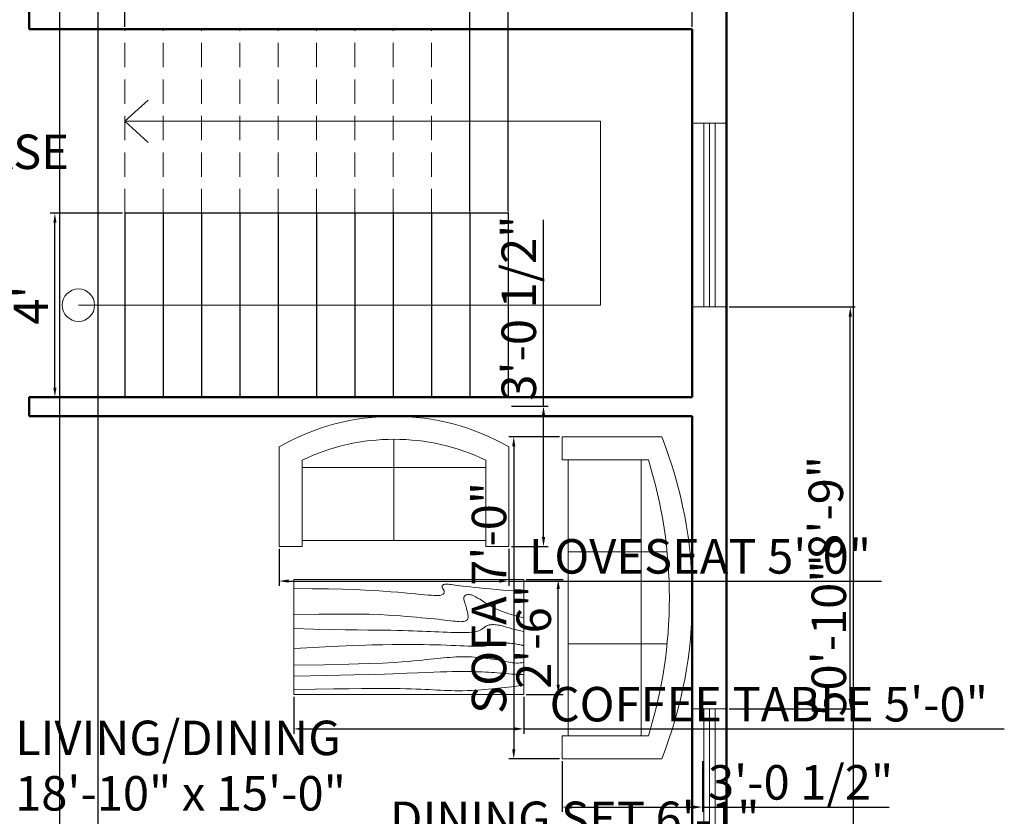
# Model space of a CAD drawing. Units: inches. Extents: x 2866 to 3545, y 873 to 1597.
# Tile 4 of 5: x 3239 to 3495, y 1172 to 1380. Entities that reach past the tile are written whole.
import ezdxf

# ---------------------------------------------------------------- set-up
doc = ezdxf.new("R2010")
doc.units = ezdxf.units.IN
doc.linetypes.add('HIDDEN', pattern=[9.525, 6.35, -3.175])
doc.layers.add('A-ANNO-DIMS', color=152, linetype='Continuous', lineweight=18, true_color=0x2776bb)
for name, color, linetype, lineweight in [('A-ANNO-SYMB', 7, 'Continuous', 18), ('A-AREA-IDEN', 7, 'Continuous', 25), ('A-FLOR-STRS', 7, 'Continuous', 25), ('A-FLOR-STRS-OVHD', 7, 'HIDDEN', 18), ('A-FURN', 8, 'Continuous', 18), ('A-GLAZ', 4, 'Continuous', 18), ('A-WALL', 7, 'Continuous', 50)]:
    doc.layers.add(name, color=color, linetype=linetype, lineweight=lineweight)
doc.styles.get("Standard").update_dxf_attribs({"font": 'arial.ttf'})
doc.dimstyles.new('ISO-25', dxfattribs={"dimtxt": 9, "dimasz": 2.5, "dimexe": 1.25, "dimexo": 0.625, "dimtad": 1, "dimdec": 0, "dimlunit": 3, "dimtxsty": 'Standard', "dimcen": 4.5, "dimadec": 0, "dimazin": 0, "dimtfac": 1, "dimtdec": 0, "dimtmove": 0, "dimatfit": 3, "dimfxl": 1, "dimarcsym": 0})

# ---------------------------------------------------------------- blocks, each defined once
blk = doc.blocks.new('Table - Rectangular Woodgrain 60 x 30 in.')
for p, q in [((0, 0), (0, -30)), ((60, 0), (0, 0)), ((60, -30), (60, 0)), ((0, -30), (60, -30))]:
    blk.add_line(p, q)
for points in [[(0, -2.4), (4.8155, -2.418), (9.0302, -2.4688), (12.709, -2.5477), (15.9167, -2.65), (18.7181, -2.7711), (21.1781, -2.9063), (23.3616, -3.0508), (25.3333, -3.2), (27.1477, -3.3495), (28.8172, -3.4958), (30.3437, -3.636), (31.7291, -3.7667), (32.9756, -3.8849), (34.0849, -3.9875), (35.059, -4.0714), (35.9, -4.1334), (36.6114, -4.1711), (37.2041, -4.1854), (37.6906, -4.1779), (38.0833, -4.15), (38.3948, -4.1034), (38.6375, -4.0396), (38.8239, -3.9602), (38.9666, -3.8667), (39.0764, -3.7608), (39.1573, -3.6448), (39.2116, -3.521), (39.2416, -3.3917), (39.2498, -3.2593), (39.2385, -3.1261), (39.21, -2.9944), (39.1666, -2.8667), (39.111, -2.7447), (39.0468, -2.6281), (38.978, -2.5163), (38.9083, -2.4083), (38.8418, -2.3035), (38.7823, -2.201), (38.7337, -2.1001), (38.7, -2), (38.6844, -1.9003), (38.6875, -1.8021), (38.7094, -1.707), (38.75, -1.6167), (38.8094, -1.5326), (38.8875, -1.4563), (38.9844, -1.3893), (39.1, -1.3333), (39.2351, -1.2896), (39.3937, -1.2583), (39.5804, -1.2396), (39.8, -1.2333), (40.057, -1.2396), (40.3562, -1.2583), (40.7023, -1.2896), (41.1, -1.3333), (41.5547, -1.3895), (42.0755, -1.4573), (42.6721, -1.5361), (43.3542, -1.625), (44.1316, -1.7233), (45.014, -1.8302), (46.0114, -1.9449), (47.1333, -2.0667), (48.3862, -2.1947), (49.7625, -2.3281), (51.2513, -2.4663), (52.8416, -2.6083), (54.5226, -2.7535), (56.2833, -2.9011), (58.1127, -3.0501), (60, -3.2)], [(0, -9.2), (6.5759, -9.0858), (11.9385, -9.0365), (16.2527, -9.0418), (19.6833, -9.0917), (22.3952, -9.1759), (24.5531, -9.2844), (26.322, -9.4069), (27.8666, -9.5333), (29.3241, -9.6553), (30.7203, -9.7719), (32.0532, -9.8837), (33.3208, -9.9917), (34.5213, -10.0965), (35.6526, -10.199), (36.7128, -10.2999), (37.7, -10.4), (38.6129, -10.4996), (39.4531, -10.5969), (40.223, -10.6895), (40.925, -10.775), (41.5613, -10.8512), (42.1344, -10.9156), (42.6465, -10.966), (43.1, -11), (43.4976, -11.0158), (43.8437, -11.0136), (44.143, -10.9942), (44.4, -10.9583), (44.6195, -10.9069), (44.8062, -10.8406), (44.9648, -10.7603), (45.1, -10.6667), (45.2155, -10.5598), (45.3114, -10.4365), (45.3871, -10.2929), (45.4416, -10.125), (45.4743, -9.929), (45.4844, -9.7011), (45.4709, -9.4371), (45.4333, -9.1333), (45.3716, -8.7883), (45.2896, -8.4104), (45.1919, -8.0107), (45.0833, -7.6), (44.9685, -7.1893), (44.8521, -6.7896), (44.7388, -6.4117), (44.6333, -6.0667), (44.54, -5.7628), (44.4614, -5.4979), (44.4001, -5.2675), (44.3583, -5.0667), (44.3384, -4.8909), (44.3427, -4.7354), (44.3736, -4.5956), (44.4333, -4.4667), (44.5236, -4.3453), (44.6427, -4.2333), (44.7884, -4.1339), (44.9583, -4.05), (45.1501, -3.9849), (45.3614, -3.9417), (45.59, -3.9234), (45.8333, -3.9333), (46.0915, -3.9749), (46.3734, -4.0531), (46.6906, -4.1736), (47.0542, -4.3417), (47.4756, -4.5629), (47.9661, -4.8427), (48.5372, -5.1866), (49.2, -5.6), (49.9676, -6.0844), (50.8594, -6.625), (51.8965, -7.2031), (53.1, -7.8), (54.491, -8.3969), (56.0906, -8.975), (57.9199, -9.5156), (60, -10)], [(0, -12.8), (5.1847, -12.9322), (9.6213, -13.0323), (13.3963, -13.1059), (16.5958, -13.1583), (19.3063, -13.1952), (21.614, -13.2219), (23.6054, -13.2439), (25.3666, -13.2667), (26.9728, -13.2947), (28.4531, -13.3281), (29.8256, -13.3663), (31.1083, -13.4083), (32.3191, -13.4535), (33.476, -13.501), (34.597, -13.5501), (35.7, -13.6), (36.7984, -13.6497), (37.8875, -13.6979), (38.9578, -13.743), (40, -13.7833), (41.0047, -13.8174), (41.9625, -13.8438), (42.864, -13.8607), (43.7, -13.8667), (44.4631, -13.8604), (45.1552, -13.8417), (45.7801, -13.8104), (46.3416, -13.7667), (46.8439, -13.7104), (47.2906, -13.6417), (47.6858, -13.5604), (48.0333, -13.4667), (48.3375, -13.3608), (48.6042, -13.2448), (48.8396, -13.121), (49.05, -12.9917), (49.2417, -12.8593), (49.4208, -12.7261), (49.5937, -12.5944), (49.7667, -12.4667), (49.9452, -12.3451), (50.1323, -12.2313), (50.3303, -12.1268), (50.5416, -12.0333), (50.7686, -11.9524), (51.0135, -11.8854), (51.2788, -11.8341), (51.5666, -11.8), (51.8785, -11.7843), (52.2116, -11.7865), (52.562, -11.8059), (52.926, -11.8417), (53.2998, -11.8931), (53.6795, -11.9594), (54.0614, -12.0397), (54.4416, -12.1333), (54.8223, -12.2401), (55.2293, -12.3625), (55.6942, -12.5037), (56.2489, -12.6667), (56.9251, -12.8547), (57.7545, -13.0708), (58.7689, -13.3182), (60, -13.6)], [(0, -18), (5.124, -17.7273), (9.6609, -17.5057), (13.6705, -17.3303), (17.2125, -17.1958), (20.3467, -17.0973), (23.1328, -17.0297), (25.6307, -16.9878), (27.9, -16.9667), (29.9928, -16.9617), (31.9302, -16.9703), (33.7254, -16.9907), (35.3917, -17.0208), (36.9423, -17.0588), (38.3906, -17.1026), (39.7499, -17.1503), (41.0333, -17.2), (42.2519, -17.2496), (43.4073, -17.2969), (44.4986, -17.3395), (45.525, -17.375), (46.4858, -17.4012), (47.3802, -17.4156), (48.2074, -17.416), (48.9667, -17.4), (49.6583, -17.3662), (50.2872, -17.3167), (50.8595, -17.2547), (51.3812, -17.1833), (51.8584, -17.1057), (52.2971, -17.025), (52.7034, -16.9443), (53.0833, -16.8667), (53.443, -16.7951), (53.789, -16.7313), (54.128, -16.6768), (54.4666, -16.6334), (54.8115, -16.6024), (55.1693, -16.5854), (55.5465, -16.5841), (55.95, -16.6), (56.3828, -16.6337), (56.8346, -16.6823), (57.2915, -16.7418), (57.7396, -16.8084), (58.165, -16.878), (58.5539, -16.9469), (58.8924, -17.0111), (59.1666, -17.0667), (59.3679, -17.1107), (59.5078, -17.1438), (59.6032, -17.1675), (59.6708, -17.1833), (59.7275, -17.193), (59.7901, -17.1979), (59.8753, -17.1998), (60, -17.2)], [(0, -22.4), (8.0098, -22.2501), (14.4094, -22.1011), (19.4168, -21.9535), (23.25, -21.8083), (26.1269, -21.6663), (28.2656, -21.5281), (29.884, -21.3947), (31.2, -21.2667), (32.3967, -21.1448), (33.5172, -21.0292), (34.5697, -20.9198), (35.5625, -20.8167), (36.5037, -20.7198), (37.4015, -20.6292), (38.2642, -20.5448), (39.1, -20.4667), (39.9164, -20.3951), (40.7187, -20.3313), (41.5117, -20.2768), (42.3, -20.2333), (43.0883, -20.2024), (43.8812, -20.1854), (44.6836, -20.1841), (45.5, -20.2), (46.3328, -20.234), (47.1747, -20.2844), (48.0163, -20.3488), (48.8479, -20.425), (49.66, -20.5106), (50.4429, -20.6031), (51.1872, -20.7004), (51.8833, -20.8), (52.5246, -20.8999), (53.1166, -20.9995), (53.6681, -21.0983), (54.1875, -21.1958), (54.6834, -21.2919), (55.1646, -21.3859), (55.6394, -21.4777), (56.1167, -21.5667), (56.6028, -21.6515), (57.0961, -21.7266), (57.5929, -21.7852), (58.0896, -21.8208), (58.5823, -21.8268), (59.0674, -21.7964), (59.5412, -21.723), (60, -21.6)], [(0, -25.2), (8.6355, -25.0504), (15.7026, -24.9031), (21.4049, -24.7606), (25.9458, -24.625), (29.529, -24.4988), (32.3578, -24.3844), (34.6359, -24.284), (36.5667, -24.2), (38.3213, -24.1341), (39.9417, -24.0854), (41.437, -24.0523), (42.8167, -24.0333), (44.0901, -24.0268), (45.2667, -24.0313), (46.3557, -24.0451), (47.3667, -24.0667), (48.309, -24.0947), (49.1928, -24.1287), (50.0284, -24.168), (50.826, -24.2125), (51.5959, -24.2617), (52.3483, -24.3151), (53.0935, -24.3725), (53.8417, -24.4334), (54.6009, -24.497), (55.3699, -24.561), (56.1454, -24.6226), (56.9239, -24.6792), (57.7021, -24.7279), (58.4764, -24.7662), (59.2435, -24.7911), (60, -24.8)], [(0, -28.8), (5.6867, -28.6681), (10.45, -28.5698), (14.407, -28.5012), (17.675, -28.4584), (20.3711, -28.4374), (22.6125, -28.4344), (24.5164, -28.4455), (26.2, -28.4667), (27.762, -28.4947), (29.2276, -28.5281), (30.6033, -28.5663), (31.8958, -28.6084), (33.1118, -28.6535), (34.2578, -28.7011), (35.3405, -28.7501), (36.3666, -28.8), (37.3443, -28.8497), (38.288, -28.8974), (39.2137, -28.9412), (40.1375, -28.9792), (41.0753, -29.0093), (42.0432, -29.0297), (43.0572, -29.0384), (44.1333, -29.0333), (45.2936, -29.0114), (46.5843, -28.9641), (48.0579, -28.8816), (49.7666, -28.7542), (51.7629, -28.5721), (54.0989, -28.3255), (56.8272, -28.0048), (60, -27.6)]]:
    blk.add_lwpolyline(points)
blk = doc.blocks.new('Sofa - Roundback Loveseat 5 ft.')
for p, q in [((0, -32.44198), (0, -5.99998)), ((-24, -33.99998), (-24, -11.46958)), ((24.00004, -33.99998), (24.00004, -11.46958)), ((-23.9998, -13.38178), (23.99986, -13.38178)), ((-24, -32.44198), (24.00004, -32.44198))]:
    blk.add_line(p, q)
for points in [[(-24, -33.99998), (-30, -33.99998), (-30, -7.99998)], [(30.00004, -7.99998), (30.00004, -33.99998), (24.00004, -33.99998)]]:
    blk.add_lwpolyline(points)
for centre, radius, start, end in [((0, -60.24998), 60.24998, 60.13715, 119.8628), ((0, -61.38438), 55.38444, 64.32083, 115.6792)]:
    blk.add_arc(centre, radius, start, end)
blk = doc.blocks.new('Sofa - Roundback 7 ft.')
for p, q in [((-12.00002, -32.4421), (-12.00003, -6.5971)), ((11.99997, -32.4421), (11.99998, -6.5971)), ((-36.000027, -34), (-36.000027, -11.4696)), ((35.99998, -34), (35.99998, -11.4696)), ((-35.999844, -13.3819), (35.9998, -13.3819)), ((-36.000027, -32.4421), (35.99998, -32.4421))]:
    blk.add_line(p, q)
for points in [[(-36.000027, -34), (-42.000027, -34), (-42.000027, -8)], [(41.99998, -8), (41.99998, -34), (35.99998, -34)]]:
    blk.add_lwpolyline(points)
for centre, radius, start, end in [((0, -114.25), 114.25, 68.43141, 111.5686), ((-0.00001, -127.1968), 121.1968, 72.72033, 107.2797)]:
    blk.add_arc(centre, radius, start, end)
blk = doc.blocks.new('*D18')
at = {"layer": 'A-ANNO-DIMS', "color": 0, "lineweight": -2, "transparency": 16777216}
for p, q in [((3265.42, 1329.69), (3246.53, 1329.69)), ((3247.78, 1284.19), (3247.78, 1327.19)), ((3265.42, 1281.69), (3246.53, 1281.69))]:
    blk.add_line(p, q, dxfattribs=at)
at = {"layer": 'A-ANNO-DIMS', "color": 0, "transparency": 16777216}
for points in [[(3247.37, 1327.19), (3248.2, 1327.19), (3247.78, 1329.69)], [(3247.37, 1284.19), (3248.2, 1284.19), (3247.78, 1281.69)]]:
    blk.add_solid(points, dxfattribs=at)
at = {"layer": 'Defpoints', "color": 0, "transparency": 16777216}
for p in [(3247.78, 1329.69), (3266.04, 1329.69), (3266.04, 1281.69)]:
    blk.add_point(p, dxfattribs=at)
at = {"layer": 'A-ANNO-DIMS', "color": 0, "transparency": 16777216, "insert": (3242.66, 1305.69), "char_height": 9, "attachment_point": 5, "rotation": 90}
blk.add_mtext("4'", dxfattribs=at)
blk = doc.blocks.new('*D19')
at = {"layer": 'A-ANNO-DIMS', "color": 0, "lineweight": -2, "transparency": 16777216}
for p, q in [((3423.67, 1523.69), (3457.33, 1523.69)), ((3456.08, 1521.19), (3456.08, 916.19)), ((3423.67, 913.69), (3457.33, 913.69))]:
    blk.add_line(p, q, dxfattribs=at)
at = {"layer": 'A-ANNO-DIMS', "color": 0, "transparency": 16777216}
for points in [[(3455.66, 1521.19), (3456.5, 1521.19), (3456.08, 1523.69)], [(3455.66, 916.19), (3456.5, 916.19), (3456.08, 913.69)]]:
    blk.add_solid(points, dxfattribs=at)
at = {"layer": 'Defpoints', "color": 0, "transparency": 16777216}
for p in [(3423.04, 1523.69), (3423.04, 913.69), (3456.08, 913.69)]:
    blk.add_point(p, dxfattribs=at)
at = {"layer": 'A-ANNO-DIMS', "color": 0, "transparency": 16777216, "insert": (3450.86, 1218.69), "char_height": 9, "attachment_point": 5, "rotation": 90}
blk.add_mtext('50\'-10"', dxfattribs=at)
blk = doc.blocks.new('WIN-48IN')
for p, q in [((0, 0), (0, 48)), ((0, 48), (9, 48)), ((3, 0), (3, 48)), ((4.5, 0), (4.5, 48)), ((6, 0), (6, 48)), ((9, 48), (9, 0)), ((9, 0), (0, 0))]:
    blk.add_line(p, q)
blk = doc.blocks.new('*D37')
at = {"layer": 'A-ANNO-DIMS', "color": 0, "lineweight": -2, "transparency": 16777216}
for p, q in [((3149.54, 1388.07), (3149.54, 1382.04)), ((3185.54, 1388.07), (3185.54, 1382.04)), ((3152.04, 1383.29), (3183.04, 1383.29)), ((3185.54, 1383.29), (3353.42, 1383.29))]:
    blk.add_line(p, q, dxfattribs=at)
at = {"layer": 'A-ANNO-DIMS', "color": 0, "transparency": 16777216}
for points in [[(3152.04, 1383.71), (3152.04, 1382.88), (3149.54, 1383.29)], [(3183.04, 1383.71), (3183.04, 1382.88), (3185.54, 1383.29)]]:
    blk.add_solid(points, dxfattribs=at)
at = {"layer": 'Defpoints', "color": 0, "transparency": 16777216}
for p in [(3149.54, 1388.69), (3185.54, 1388.69), (3185.54, 1383.29)]:
    blk.add_point(p, dxfattribs=at)
at = {"layer": 'A-ANNO-DIMS', "color": 0, "transparency": 16777216, "insert": (3270.73, 1388.58), "char_height": 9, "attachment_point": 5}
blk.add_mtext('BEDROOM DOOR 3\'-0" TYP.', dxfattribs=at)
blk = doc.blocks.new('*D47')
at = {"layer": 'A-ANNO-DIMS', "color": 0, "lineweight": -2, "transparency": 16777216}
for p, q in [((3310.1, 1203.48), (3310.1, 1193.86)), ((3370.1, 1203.48), (3370.1, 1193.86)), ((3312.6, 1195.11), (3367.6, 1195.11)), ((3370.1, 1195.11), (3495.47, 1195.11))]:
    blk.add_line(p, q, dxfattribs=at)
at = {"layer": 'A-ANNO-DIMS', "color": 0, "transparency": 16777216}
for points in [[(3312.6, 1195.53), (3312.6, 1194.69), (3310.1, 1195.11)], [(3367.6, 1195.53), (3367.6, 1194.69), (3370.1, 1195.11)]]:
    blk.add_solid(points, dxfattribs=at)
at = {"layer": 'Defpoints', "color": 0, "transparency": 16777216}
for p in [(3310.1, 1204.11), (3370.1, 1204.11), (3370.1, 1195.11)]:
    blk.add_point(p, dxfattribs=at)
at = {"layer": 'A-ANNO-DIMS', "color": 0, "transparency": 16777216, "insert": (3434.03, 1200.39), "char_height": 9, "attachment_point": 5}
blk.add_mtext('COFFEE TABLE 5\'-0"', dxfattribs=at)
blk = doc.blocks.new('*D48')
at = {"layer": 'A-ANNO-DIMS', "color": 0, "lineweight": -2, "transparency": 16777216}
for p, q in [((3370.72, 1234.11), (3380.35, 1234.11)), ((3379.1, 1206.61), (3379.1, 1231.61)), ((3370.72, 1204.11), (3380.35, 1204.11))]:
    blk.add_line(p, q, dxfattribs=at)
at = {"layer": 'A-ANNO-DIMS', "color": 0, "transparency": 16777216}
for points in [[(3378.68, 1231.61), (3379.51, 1231.61), (3379.1, 1234.11)], [(3378.68, 1206.61), (3379.51, 1206.61), (3379.1, 1204.11)]]:
    blk.add_solid(points, dxfattribs=at)
at = {"layer": 'Defpoints', "color": 0, "transparency": 16777216}
for p in [(3370.1, 1234.11), (3379.1, 1234.11), (3370.1, 1204.11)]:
    blk.add_point(p, dxfattribs=at)
at = {"layer": 'A-ANNO-DIMS', "color": 0, "transparency": 16777216, "insert": (3373.87, 1219.11), "char_height": 9, "attachment_point": 5, "rotation": 90}
blk.add_mtext('2\'-6"', dxfattribs=at)
blk = doc.blocks.new('*D49')
at = {"layer": 'A-ANNO-DIMS', "color": 0, "lineweight": -2, "transparency": 16777216}
for p, q in [((3306.25, 1242.07), (3306.25, 1232.44)), ((3366.25, 1242.07), (3366.25, 1232.44)), ((3308.75, 1233.69), (3363.75, 1233.69)), ((3366.25, 1233.69), (3463.4, 1233.69))]:
    blk.add_line(p, q, dxfattribs=at)
at = {"layer": 'A-ANNO-DIMS', "color": 0, "transparency": 16777216}
for points in [[(3308.75, 1234.11), (3308.75, 1233.28), (3306.25, 1233.69)], [(3363.75, 1234.11), (3363.75, 1233.28), (3366.25, 1233.69)]]:
    blk.add_solid(points, dxfattribs=at)
at = {"layer": 'Defpoints', "color": 0, "transparency": 16777216}
for p in [(3306.25, 1242.69), (3366.25, 1242.69), (3366.25, 1233.69)]:
    blk.add_point(p, dxfattribs=at)
at = {"layer": 'A-ANNO-DIMS', "color": 0, "transparency": 16777216, "insert": (3416.07, 1238.97), "char_height": 9, "attachment_point": 5}
blk.add_mtext('LOVESEAT 5\'-0"', dxfattribs=at)
blk = doc.blocks.new('*D50')
at = {"layer": 'A-ANNO-DIMS', "color": 0, "lineweight": -2, "transparency": 16777216}
for p, q in [((3375.25, 1279.36), (3375.25, 1328)), ((3366.87, 1279.36), (3376.5, 1279.36)), ((3375.25, 1245.19), (3375.25, 1276.86)), ((3366.87, 1242.69), (3376.5, 1242.69))]:
    blk.add_line(p, q, dxfattribs=at)
at = {"layer": 'A-ANNO-DIMS', "color": 0, "transparency": 16777216}
for points in [[(3374.83, 1276.86), (3375.67, 1276.86), (3375.25, 1279.36)], [(3374.83, 1245.19), (3375.67, 1245.19), (3375.25, 1242.69)]]:
    blk.add_solid(points, dxfattribs=at)
at = {"layer": 'Defpoints', "color": 0, "transparency": 16777216}
for p in [(3366.25, 1279.36), (3375.25, 1279.36), (3366.25, 1242.69)]:
    blk.add_point(p, dxfattribs=at)
at = {"layer": 'A-ANNO-DIMS', "color": 0, "transparency": 16777216, "insert": (3369.97, 1304.93), "char_height": 9, "attachment_point": 5, "rotation": 90}
blk.add_mtext('3\'-0 1/2"', dxfattribs=at)
blk = doc.blocks.new('*D53')
at = {"layer": 'A-ANNO-DIMS', "color": 0, "lineweight": -2, "transparency": 16777216}
for p, q in [((3257.81, 1154.88), (3257.81, 1166.46)), ((3330.83, 1154.88), (3330.83, 1166.46)), ((3260.31, 1165.21), (3328.33, 1165.21)), ((3330.83, 1165.21), (3433.5, 1165.21))]:
    blk.add_line(p, q, dxfattribs=at)
at = {"layer": 'A-ANNO-DIMS', "color": 0, "transparency": 16777216}
for points in [[(3260.31, 1165.62), (3260.31, 1164.79), (3257.81, 1165.21)], [(3328.33, 1165.62), (3328.33, 1164.79), (3330.83, 1165.21)]]:
    blk.add_solid(points, dxfattribs=at)
at = {"layer": 'Defpoints', "color": 0, "transparency": 16777216}
for p in [(3330.83, 1165.21), (3257.81, 1154.25), (3330.83, 1154.25)]:
    blk.add_point(p, dxfattribs=at)
at = {"layer": 'A-ANNO-DIMS', "color": 0, "transparency": 16777216, "insert": (3383.42, 1170.48), "char_height": 9, "attachment_point": 5}
blk.add_mtext('DINING SET 6\'-1"', dxfattribs=at)
blk = doc.blocks.new('*D55')
at = {"layer": 'A-ANNO-DIMS', "color": 0, "lineweight": -2, "transparency": 16777216}
for p, q in [((3379.47, 1271.31), (3366.24, 1271.31)), ((3367.49, 1268.81), (3367.49, 1189.81)), ((3379.47, 1187.31), (3366.24, 1187.31))]:
    blk.add_line(p, q, dxfattribs=at)
at = {"layer": 'A-ANNO-DIMS', "color": 0, "transparency": 16777216}
for points in [[(3367.08, 1268.81), (3367.91, 1268.81), (3367.49, 1271.31)], [(3367.08, 1189.81), (3367.91, 1189.81), (3367.49, 1187.31)]]:
    blk.add_solid(points, dxfattribs=at)
at = {"layer": 'Defpoints', "color": 0, "transparency": 16777216}
for p in [(3380.09, 1271.31), (3367.49, 1187.31), (3380.09, 1187.31)]:
    blk.add_point(p, dxfattribs=at)
at = {"layer": 'A-ANNO-DIMS', "color": 0, "transparency": 16777216, "insert": (3362.21, 1229.31), "char_height": 9, "attachment_point": 5, "rotation": 90}
blk.add_mtext('SOFA 7\'-0"', dxfattribs=at)
blk = doc.blocks.new('*D56')
at = {"layer": 'A-ANNO-DIMS', "color": 0, "lineweight": -2, "transparency": 16777216}
for p, q in [((3380.09, 1186.68), (3380.09, 1173.46)), ((3416.76, 1186.68), (3416.76, 1173.46)), ((3382.59, 1174.71), (3414.26, 1174.71)), ((3416.76, 1174.71), (3465.4, 1174.71))]:
    blk.add_line(p, q, dxfattribs=at)
at = {"layer": 'A-ANNO-DIMS', "color": 0, "transparency": 16777216}
for points in [[(3382.59, 1175.12), (3382.59, 1174.29), (3380.09, 1174.71)], [(3414.26, 1175.12), (3414.26, 1174.29), (3416.76, 1174.71)]]:
    blk.add_solid(points, dxfattribs=at)
at = {"layer": 'Defpoints', "color": 0, "transparency": 16777216}
for p in [(3380.09, 1187.31), (3416.76, 1187.31), (3416.76, 1174.71)]:
    blk.add_point(p, dxfattribs=at)
at = {"layer": 'A-ANNO-DIMS', "color": 0, "transparency": 16777216, "insert": (3442.33, 1179.99), "char_height": 9, "attachment_point": 5}
blk.add_mtext('3\'-0 1/2"', dxfattribs=at)
blk = doc.blocks.new('*D73')
at = {"layer": 'A-ANNO-DIMS', "color": 0, "lineweight": -2, "transparency": 16777216}
for p, q in [((3423.67, 1305.22), (3456.54, 1305.22)), ((3455.29, 1202.87), (3455.29, 1302.72)), ((3423.67, 1200.37), (3456.54, 1200.37))]:
    blk.add_line(p, q, dxfattribs=at)
at = {"layer": 'A-ANNO-DIMS', "color": 0, "transparency": 16777216}
for points in [[(3454.88, 1302.72), (3455.71, 1302.72), (3455.29, 1305.22)], [(3454.88, 1202.87), (3455.71, 1202.87), (3455.29, 1200.37)]]:
    blk.add_solid(points, dxfattribs=at)
at = {"layer": 'Defpoints', "color": 0, "transparency": 16777216}
for p in [(3423.04, 1305.22), (3455.29, 1305.22), (3423.04, 1200.37)]:
    blk.add_point(p, dxfattribs=at)
at = {"layer": 'A-ANNO-DIMS', "color": 0, "transparency": 16777216, "insert": (3450.07, 1252.8), "char_height": 9, "attachment_point": 5, "rotation": 90}
blk.add_mtext('8\'-9"', dxfattribs=at)
blk = doc.blocks.new('*D80')
at = {"layer": 'A-ANNO-DIMS', "color": 0, "lineweight": -2, "transparency": 16777216}
for p, q in [((3249.04, 1088.32), (3249.04, 1557.19)), ((3259.04, 1088.32), (3259.04, 1557.19)), ((3251.54, 1555.94), (3256.54, 1555.94)), ((3259.04, 1555.94), (3293.71, 1555.94))]:
    blk.add_line(p, q, dxfattribs=at)
at = {"layer": 'A-ANNO-DIMS', "color": 0, "transparency": 16777216}
for points in [[(3251.54, 1556.36), (3251.54, 1555.53), (3249.04, 1555.94)], [(3256.54, 1556.36), (3256.54, 1555.53), (3259.04, 1555.94)]]:
    blk.add_solid(points, dxfattribs=at)
at = {"layer": 'Defpoints', "color": 0, "transparency": 16777216}
for p in [(3259.04, 1555.94), (3249.04, 1087.69), (3259.04, 1087.69)]:
    blk.add_point(p, dxfattribs=at)
at = {"layer": 'A-ANNO-DIMS', "color": 0, "transparency": 16777216, "insert": (3277.63, 1561.16), "char_height": 9, "attachment_point": 5}
blk.add_mtext('0\'-10"', dxfattribs=at)
blk = doc.blocks.new('*D81')
at = {"layer": 'A-ANNO-DIMS', "color": 0, "lineweight": -2, "transparency": 16777216}
for p, q in [((3266.04, 1378.32), (3266.04, 1557.19)), ((3366.04, 1378.32), (3366.04, 1557.19)), ((3268.54, 1555.94), (3363.54, 1555.94))]:
    blk.add_line(p, q, dxfattribs=at)
at = {"layer": 'A-ANNO-DIMS', "color": 0, "transparency": 16777216}
for points in [[(3268.54, 1556.36), (3268.54, 1555.53), (3266.04, 1555.94)], [(3363.54, 1556.36), (3363.54, 1555.53), (3366.04, 1555.94)]]:
    blk.add_solid(points, dxfattribs=at)
at = {"layer": 'Defpoints', "color": 0, "transparency": 16777216}
for p in [(3366.04, 1555.94), (3266.04, 1377.69), (3366.04, 1377.69)]:
    blk.add_point(p, dxfattribs=at)
at = {"layer": 'A-ANNO-DIMS', "color": 0, "transparency": 16777216, "insert": (3316.04, 1561.16), "char_height": 9, "attachment_point": 5}
blk.add_mtext('8\'-4"', dxfattribs=at)
blk = doc.blocks.new('*D82')
at = {"layer": 'A-ANNO-DIMS', "color": 0, "lineweight": -2, "transparency": 16777216}
for p, q in [((3366.04, 1378.32), (3366.04, 1557.19)), ((3414.04, 1378.32), (3414.04, 1557.19)), ((3368.54, 1555.94), (3411.54, 1555.94))]:
    blk.add_line(p, q, dxfattribs=at)
at = {"layer": 'A-ANNO-DIMS', "color": 0, "transparency": 16777216}
for points in [[(3368.54, 1556.36), (3368.54, 1555.53), (3366.04, 1555.94)], [(3411.54, 1556.36), (3411.54, 1555.53), (3414.04, 1555.94)]]:
    blk.add_solid(points, dxfattribs=at)
at = {"layer": 'Defpoints', "color": 0, "transparency": 16777216}
for p in [(3414.04, 1555.94), (3366.04, 1377.69), (3414.04, 1377.69)]:
    blk.add_point(p, dxfattribs=at)
at = {"layer": 'A-ANNO-DIMS', "color": 0, "transparency": 16777216, "insert": (3390.04, 1561.16), "char_height": 9, "attachment_point": 5}
blk.add_mtext('4\'-0"', dxfattribs=at)
blk = doc.blocks.new('*D83')
at = {"layer": 'A-ANNO-DIMS', "color": 0, "lineweight": -2, "transparency": 16777216}
for p, q in [((3356.04, 1330.32), (3356.04, 1557.19)), ((3366.04, 1330.32), (3366.04, 1557.19)), ((3358.54, 1555.94), (3363.54, 1555.94)), ((3366.04, 1555.94), (3400.71, 1555.94))]:
    blk.add_line(p, q, dxfattribs=at)
at = {"layer": 'A-ANNO-DIMS', "color": 0, "transparency": 16777216}
for points in [[(3358.54, 1556.36), (3358.54, 1555.53), (3356.04, 1555.94)], [(3363.54, 1556.36), (3363.54, 1555.53), (3366.04, 1555.94)]]:
    blk.add_solid(points, dxfattribs=at)
at = {"layer": 'Defpoints', "color": 0, "transparency": 16777216}
for p in [(3366.04, 1555.94), (3356.04, 1329.69), (3366.04, 1329.69)]:
    blk.add_point(p, dxfattribs=at)
at = {"layer": 'A-ANNO-DIMS', "color": 0, "transparency": 16777216, "insert": (3384.63, 1561.16), "char_height": 9, "attachment_point": 5}
blk.add_mtext('0\'-10"', dxfattribs=at)

msp = doc.modelspace()

# ---------------------------------------------------------------- linework, layer by layer
at = {"layer": 'A-ANNO-SYMB'}
for p, q in [((3266.04, 1353.69), (3272.15, 1359.21)), ((3390.12, 1353.69), (3266.04, 1353.69)), ((3266.04, 1353.69), (3272.15, 1348.17)), ((3390.12, 1305.69), (3390.12, 1353.69)), ((3266.04, 1305.69), (3253.92, 1305.69)), ((3266.04, 1305.69), (3390.12, 1305.69))]:
    msp.add_line(p, q, dxfattribs=at)
msp.add_circle((3253.92, 1305.69), 4.23, dxfattribs=at)
at = {"layer": 'A-FLOR-STRS'}
for p, q in [((3366.04, 1329.69), (3266.04, 1329.69)), ((3266.04, 1329.69), (3266.04, 1281.69)), ((3276.04, 1329.69), (3276.04, 1281.69)), ((3286.04, 1329.69), (3286.04, 1281.69)), ((3296.04, 1329.69), (3296.04, 1281.69)), ((3306.04, 1329.69), (3306.04, 1281.69)), ((3316.04, 1329.69), (3316.04, 1281.69)), ((3326.04, 1329.69), (3326.04, 1281.69)), ((3336.04, 1329.69), (3336.04, 1281.69)), ((3346.04, 1329.69), (3346.04, 1281.69)), ((3356.04, 1329.69), (3356.04, 1281.69)), ((3366.04, 1329.69), (3366.04, 1281.69))]:
    msp.add_line(p, q, dxfattribs=at)
at = {"layer": 'A-FLOR-STRS-OVHD'}
for p, q in [((3266.04, 1329.69), (3266.04, 1377.69)), ((3276.04, 1329.69), (3276.04, 1377.69)), ((3286.04, 1329.69), (3286.04, 1377.69)), ((3296.04, 1329.69), (3296.04, 1377.69)), ((3306.04, 1329.69), (3306.04, 1377.69)), ((3316.04, 1329.69), (3316.04, 1377.69)), ((3326.04, 1329.69), (3326.04, 1377.69)), ((3336.04, 1329.69), (3336.04, 1377.69)), ((3346.04, 1329.69), (3346.04, 1377.69)), ((3356.04, 1329.69), (3356.04, 1377.69)), ((3366.04, 1329.69), (3366.04, 1377.69))]:
    msp.add_line(p, q, dxfattribs=at)
at = {"layer": 'A-WALL'}
for p, q in [((3423.04, 1523.69), (3423.04, 913.69)), ((3241.04, 1382.69), (3241.04, 1377.69)), ((3241.04, 1377.69), (3414.04, 1377.69)), ((3414.04, 1377.69), (3414.04, 1281.69)), ((3241.04, 1281.69), (3414.04, 1281.69)), ((3241.04, 1281.69), (3241.04, 1276.69)), ((3241.04, 1276.69), (3414.04, 1276.69)), ((3414.04, 1276.69), (3414.04, 1096.69))]:
    msp.add_line(p, q, dxfattribs=at)

# ---------------------------------------------------------------- block references
at = {"layer": 'A-FURN'}
for name, p in [('Sofa - Roundback Loveseat 5 ft.', (3336.25, 1276.69)), ('Table - Rectangular Woodgrain 60 x 30 in.', (3310.1, 1234.11))]:
    msp.add_blockref(name, p, dxfattribs=at)
at = {"layer": 'A-FURN', "rotation": 270}
msp.add_blockref('Sofa - Roundback 7 ft.', (3414.09, 1229.31), dxfattribs=at)
at = {"layer": 'A-GLAZ'}
for p in [(3414.04, 1305.22), (3414.04, 1152.37)]:
    msp.add_blockref('WIN-48IN', p, dxfattribs=at)

# ---------------------------------------------------------------- texts
at = {"layer": 'A-AREA-IDEN'}
for s, p in [('STAIRCASE', (3188.07, 1341.21)), ('LIVING/DINING', (3237.41, 1188.26)), ('18\'-10" x 15\'-0"', (3237.41, 1173.8))]:
    msp.add_text(s, height=9, dxfattribs=at).set_placement(p)

# ---------------------------------------------------------------- dimensions: what is measured, and where the dimension line sits
at = {"layer": 'A-ANNO-DIMS'}
for base, p1, p2, picture, middle in [((3259.04, 1555.94), (3249.04, 1087.69), (3259.04, 1087.69), '*D80', (3277.63, 1561.16)), ((3366.04, 1555.94), (3266.04, 1377.69), (3366.04, 1377.69), '*D81', (3316.04, 1561.16)), ((3366.04, 1555.94), (3356.04, 1329.69), (3366.04, 1329.69), '*D83', (3384.63, 1561.16)), ((3414.04, 1555.94), (3366.04, 1377.69), (3414.04, 1377.69), '*D82', (3390.04, 1561.16)), ((3416.76, 1174.71), (3380.09, 1187.31), (3416.76, 1187.31), '*D56', (3442.33, 1179.99))]:
    dim = msp.add_linear_dim(base=base, p1=p1, p2=p2, dimstyle='ISO-25', override={"dimdec": 1, "dimlfac": 1, "dimrnd": 0, "dimzin": 1, "dimdsep": 46, "dimlunit": 4, "dimfrac": 2}, dxfattribs=at)
    dim.commit()
    dim.dimension.update_dxf_attribs({"geometry": picture, "text_midpoint": middle})
for base, p1, p2, override, picture, middle in [((3456.08, 913.69), (3423.04, 1523.69), (3423.04, 913.69), {"dimclrd": 0, "dimclre": 0, "dimclrt": 0}, '*D19', (3450.86, 1218.69)), ((3247.78, 1329.69), (3266.04, 1281.69), (3266.04, 1329.69), {"dimclrd": 0, "dimclre": 0, "dimclrt": 0}, '*D18', (3242.66, 1305.69)), ((3375.25, 1279.36), (3366.25, 1242.69), (3366.25, 1279.36), {"dimdec": 1, "dimlfac": 1, "dimrnd": 0, "dimzin": 1, "dimdsep": 46, "dimlunit": 4, "dimfrac": 2}, '*D50', (3369.97, 1304.93)), ((3455.2917, 1305.2168), (3423.0417, 1200.3745), (3423.0417, 1305.2168), {"dimdec": 1, "dimlfac": 1, "dimrnd": 0, "dimzin": 1, "dimdsep": 46, "dimlunit": 4, "dimfrac": 2}, '*D73', (3450.0716, 1252.7956)), ((3379.1, 1234.11), (3370.1, 1204.11), (3370.1, 1234.11), {"dimdec": 1, "dimlfac": 1, "dimrnd": 0, "dimzin": 1, "dimdsep": 46, "dimlunit": 4, "dimfrac": 2}, '*D48', (3373.87, 1219.11))]:
    dim = msp.add_linear_dim(base=base, p1=p1, p2=p2, angle=90, dimstyle='ISO-25', override=override, dxfattribs=at)
    dim.commit()
    dim.dimension.update_dxf_attribs({"geometry": picture, "text_midpoint": middle})
for base, p1, p2, text, picture, middle in [((3185.54, 1383.29), (3149.54, 1388.69), (3185.54, 1388.69), 'BEDROOM DOOR <> TYP.', '*D37', (3270.73, 1388.58)), ((3366.25, 1233.69), (3306.25, 1242.69), (3366.25, 1242.69), 'LOVESEAT <>', '*D49', (3416.07, 1238.97)), ((3370.1, 1195.11), (3310.1, 1204.11), (3370.1, 1204.11), 'COFFEE TABLE <>', '*D47', (3434.03, 1200.39)), ((3330.83, 1165.21), (3257.81, 1154.25), (3330.83, 1154.25), 'DINING SET <>', '*D53', (3383.42, 1170.48))]:
    dim = msp.add_linear_dim(base=base, p1=p1, p2=p2, text=text, dimstyle='ISO-25', override={"dimdec": 1, "dimlfac": 1, "dimrnd": 0, "dimzin": 1, "dimdsep": 46, "dimlunit": 4, "dimfrac": 2}, dxfattribs=at)
    dim.commit()
    dim.dimension.update_dxf_attribs({"geometry": picture, "text_midpoint": middle})
dim = msp.add_linear_dim(base=(3367.49, 1187.31), p1=(3380.09, 1271.31), p2=(3380.09, 1187.31), angle=270, text='SOFA <>', dimstyle='ISO-25', override={"dimdec": 1, "dimlfac": 1, "dimrnd": 0, "dimzin": 1, "dimdsep": 46, "dimlunit": 4, "dimfrac": 2}, dxfattribs=at)
dim.commit()
dim.dimension.update_dxf_attribs({"geometry": '*D55', "text_midpoint": (3362.21, 1229.31)})

doc.saveas('drawing.dxf')
